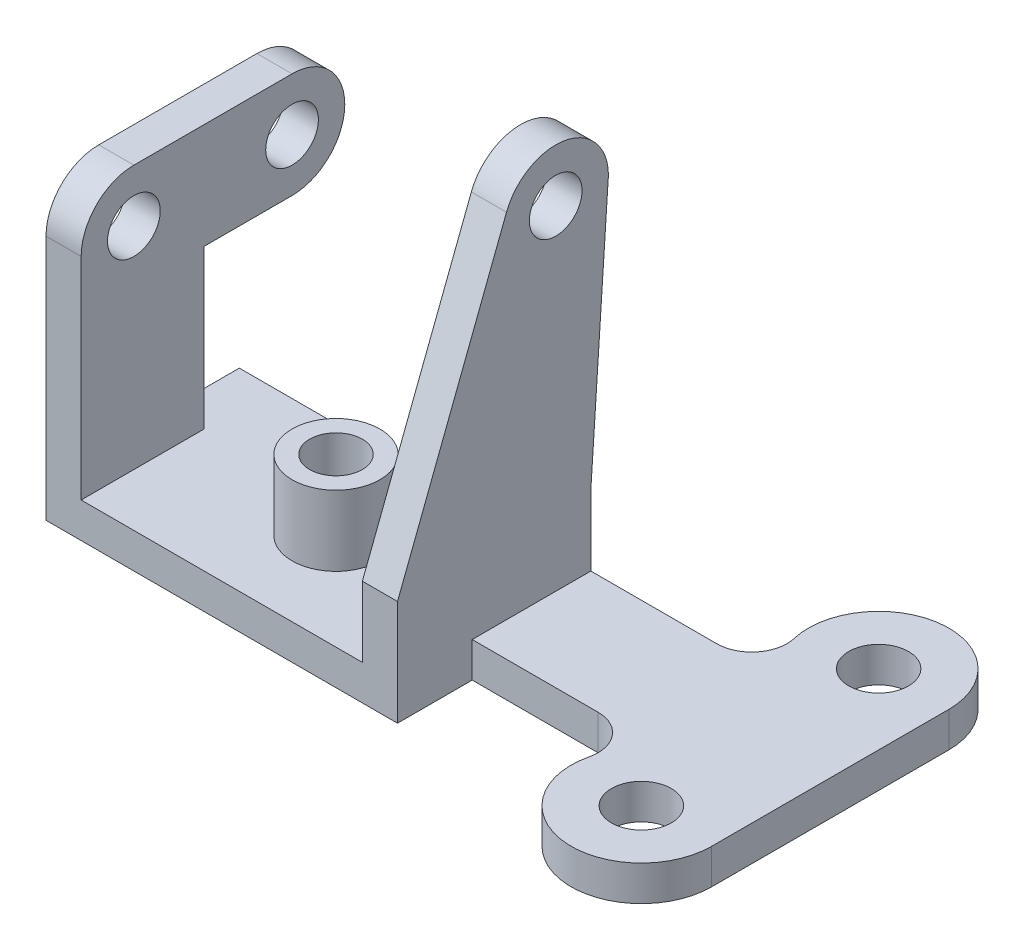
ISO-10303-21;
HEADER;
FILE_DESCRIPTION(('STEP AP214'),'2;1');
FILE_NAME('part.step','',(''),(''),'','','');
FILE_SCHEMA(('AUTOMOTIVE_DESIGN { 1 0 10303 214 1 1 1 1 }'));
ENDSEC;
DATA;
#1=APPLICATION_CONTEXT('core data for automotive mechanical design processes');
#2=APPLICATION_PROTOCOL_DEFINITION('international standard','automotive_design',2000,#1);
#3=PRODUCT_CONTEXT('',#1,'mechanical');
#4=PRODUCT('Part','Part','',(#3));
#5=PRODUCT_RELATED_PRODUCT_CATEGORY('part','',(#4));
#6=PRODUCT_DEFINITION_FORMATION('','',#4);
#7=PRODUCT_DEFINITION_CONTEXT('part definition',#1,'design');
#8=PRODUCT_DEFINITION('design','',#6,#7);
#9=PRODUCT_DEFINITION_SHAPE('','',#8);
#10=(LENGTH_UNIT() NAMED_UNIT(*) SI_UNIT(.MILLI.,.METRE.));
#11=(NAMED_UNIT(*) PLANE_ANGLE_UNIT() SI_UNIT($,.RADIAN.));
#12=(NAMED_UNIT(*) SI_UNIT($,.STERADIAN.) SOLID_ANGLE_UNIT());
#13=UNCERTAINTY_MEASURE_WITH_UNIT(LENGTH_MEASURE(1.E-05),#10,'distance_accuracy_value','');
#14=(GEOMETRIC_REPRESENTATION_CONTEXT(3) GLOBAL_UNCERTAINTY_ASSIGNED_CONTEXT((#13)) GLOBAL_UNIT_ASSIGNED_CONTEXT((#10,
#11,#12)) REPRESENTATION_CONTEXT('',''));
#15=CARTESIAN_POINT('',(0.,0.,0.));
#16=DIRECTION('',(0.,0.,1.));
#17=DIRECTION('',(1.,0.,0.));
#18=AXIS2_PLACEMENT_3D('',#15,#16,#17);
#19=CARTESIAN_POINT('',(0.,20.,0.));
#20=DIRECTION('',(0.,1.,0.));
#21=DIRECTION('',(0.,0.,1.));
#22=AXIS2_PLACEMENT_3D('',#19,#20,#21);
#23=PLANE('',#22);
#24=CARTESIAN_POINT('',(9.99999999999997,20.,0.));
#25=DIRECTION('',(0.,1.,0.));
#26=DIRECTION('',(0.,0.,1.));
#27=AXIS2_PLACEMENT_3D('',#24,#25,#26);
#28=CIRCLE('',#27,25.);
#29=CARTESIAN_POINT('',(9.99999999999997,20.,25.));
#30=VERTEX_POINT('',#29);
#31=EDGE_CURVE('E805',#30,#30,#28,.T.);
#32=ORIENTED_EDGE('',*,*,#31,.F.);
#33=EDGE_LOOP('',(#32));
#34=FACE_BOUND('',#33,.T.);
#35=DIRECTION('',(1.,0.,0.));
#36=VECTOR('',#35,1.);
#37=CARTESIAN_POINT('',(-100.,20.,55.));
#38=LINE('',#37,#36);
#39=CARTESIAN_POINT('',(-80.,20.,55.));
#40=VERTEX_POINT('',#39);
#41=CARTESIAN_POINT('',(80.,20.,55.));
#42=VERTEX_POINT('',#41);
#43=EDGE_CURVE('E68',#40,#42,#38,.T.);
#44=ORIENTED_EDGE('',*,*,#43,.T.);
#45=DIRECTION('',(0.,0.,1.));
#46=VECTOR('',#45,1.);
#47=CARTESIAN_POINT('',(80.,20.,0.));
#48=LINE('',#47,#46);
#49=CARTESIAN_POINT('',(80.,20.,-55.));
#50=VERTEX_POINT('',#49);
#51=EDGE_CURVE('E61',#50,#42,#48,.T.);
#52=ORIENTED_EDGE('',*,*,#51,.F.);
#53=DIRECTION('',(-1.,0.,0.));
#54=VECTOR('',#53,1.);
#55=CARTESIAN_POINT('',(-100.,20.,-55.));
#56=LINE('',#55,#54);
#57=CARTESIAN_POINT('',(-100.,20.,-55.));
#58=VERTEX_POINT('',#57);
#59=EDGE_CURVE('E372',#50,#58,#56,.T.);
#60=ORIENTED_EDGE('',*,*,#59,.T.);
#61=DIRECTION('',(0.,0.,1.));
#62=VECTOR('',#61,1.);
#63=CARTESIAN_POINT('',(-100.,20.,-55.));
#64=LINE('',#63,#62);
#65=CARTESIAN_POINT('',(-100.,20.,-15.));
#66=VERTEX_POINT('',#65);
#67=EDGE_CURVE('E373',#58,#66,#64,.T.);
#68=ORIENTED_EDGE('',*,*,#67,.T.);
#69=DIRECTION('',(-1.,0.,0.));
#70=VECTOR('',#69,1.);
#71=CARTESIAN_POINT('',(0.,20.,-15.));
#72=LINE('',#71,#70);
#73=CARTESIAN_POINT('',(-80.,20.,-15.));
#74=VERTEX_POINT('',#73);
#75=EDGE_CURVE('E303',#74,#66,#72,.T.);
#76=ORIENTED_EDGE('',*,*,#75,.F.);
#77=DIRECTION('',(0.,0.,1.));
#78=VECTOR('',#77,1.);
#79=CARTESIAN_POINT('',(-80.,20.,0.));
#80=LINE('',#79,#78);
#81=EDGE_CURVE('E291',#74,#40,#80,.T.);
#82=ORIENTED_EDGE('',*,*,#81,.T.);
#83=EDGE_LOOP('',(#44,#52,#60,#68,#76,#82));
#84=FACE_BOUND('',#83,.T.);
#85=ADVANCED_FACE('F50',(#34,#84),#23,.T.);
#86=CARTESIAN_POINT('',(100.,20.,-55.));
#87=DIRECTION('',(-1.,0.,0.));
#88=DIRECTION('',(0.,0.,1.));
#89=AXIS2_PLACEMENT_3D('',#86,#87,#88);
#90=PLANE('',#89);
#91=DIRECTION('',(0.,0.,-1.));
#92=VECTOR('',#91,1.);
#93=CARTESIAN_POINT('',(100.,0.,-55.));
#94=LINE('',#93,#92);
#95=CARTESIAN_POINT('',(100.,0.,55.));
#96=VERTEX_POINT('',#95);
#97=CARTESIAN_POINT('',(100.,0.,12.5));
#98=VERTEX_POINT('',#97);
#99=EDGE_CURVE('E358',#96,#98,#94,.T.);
#100=ORIENTED_EDGE('',*,*,#99,.T.);
#101=DIRECTION('',(0.,1.,0.));
#102=VECTOR('',#101,1.);
#103=CARTESIAN_POINT('',(100.,0.,12.5));
#104=LINE('',#103,#102);
#105=CARTESIAN_POINT('',(100.,20.,12.5));
#106=VERTEX_POINT('',#105);
#107=EDGE_CURVE('E336',#98,#106,#104,.T.);
#108=ORIENTED_EDGE('',*,*,#107,.T.);
#109=DIRECTION('',(0.,0.,1.));
#110=VECTOR('',#109,1.);
#111=CARTESIAN_POINT('',(100.,20.,0.));
#112=LINE('',#111,#110);
#113=CARTESIAN_POINT('',(100.,20.,-55.));
#114=VERTEX_POINT('',#113);
#115=EDGE_CURVE('E240',#114,#106,#112,.T.);
#116=ORIENTED_EDGE('',*,*,#115,.F.);
#117=DIRECTION('',(0.,1.,0.));
#118=VECTOR('',#117,1.);
#119=CARTESIAN_POINT('',(100.,0.,-55.));
#120=LINE('',#119,#118);
#121=CARTESIAN_POINT('',(100.,60.,-55.));
#122=VERTEX_POINT('',#121);
#123=EDGE_CURVE('E217',#114,#122,#120,.T.);
#124=ORIENTED_EDGE('',*,*,#123,.T.);
#125=DIRECTION('',(0.,0.997785157856609,-0.0665190105237738));
#126=VECTOR('',#125,1.);
#127=CARTESIAN_POINT('',(100.,-3.38495575221238,-50.7743362831858));
#128=LINE('',#127,#126);
#129=CARTESIAN_POINT('',(100.,210.,-65.));
#130=VERTEX_POINT('',#129);
#131=EDGE_CURVE('E227',#122,#130,#128,.T.);
#132=ORIENTED_EDGE('',*,*,#131,.T.);
#133=CARTESIAN_POINT('',(100.,210.,-35.));
#134=DIRECTION('',(1.,0.,0.));
#135=DIRECTION('',(0.,0.,-1.));
#136=AXIS2_PLACEMENT_3D('',#133,#134,#135);
#137=CIRCLE('',#136,30.);
#138=CARTESIAN_POINT('',(100.,220.794430534954,-7.00928244174394));
#139=VERTEX_POINT('',#138);
#140=EDGE_CURVE('E194',#130,#139,#137,.T.);
#141=ORIENTED_EDGE('',*,*,#140,.T.);
#142=DIRECTION('',(0.,0.933023918608534,-0.35981435116512));
#143=VECTOR('',#142,1.);
#144=CARTESIAN_POINT('',(100.,26.2323288125243,68.0222735519993));
#145=LINE('',#144,#143);
#146=CARTESIAN_POINT('',(100.,60.,55.));
#147=VERTEX_POINT('',#146);
#148=EDGE_CURVE('E232',#147,#139,#145,.T.);
#149=ORIENTED_EDGE('',*,*,#148,.F.);
#150=DIRECTION('',(0.,-1.,0.));
#151=VECTOR('',#150,1.);
#152=CARTESIAN_POINT('',(100.,20.,55.));
#153=LINE('',#152,#151);
#154=EDGE_CURVE('E380',#147,#96,#153,.T.);
#155=ORIENTED_EDGE('',*,*,#154,.T.);
#156=EDGE_LOOP('',(#100,#108,#116,#124,#132,#141,#149,#155));
#157=FACE_BOUND('',#156,.T.);
#158=CARTESIAN_POINT('',(100.,210.,-35.));
#159=DIRECTION('',(1.,0.,0.));
#160=DIRECTION('',(0.,0.,-1.));
#161=AXIS2_PLACEMENT_3D('',#158,#159,#160);
#162=CIRCLE('',#161,15.);
#163=CARTESIAN_POINT('',(100.,210.,-50.));
#164=VERTEX_POINT('',#163);
#165=EDGE_CURVE('E230',#164,#164,#162,.T.);
#166=ORIENTED_EDGE('',*,*,#165,.F.);
#167=EDGE_LOOP('',(#166));
#168=FACE_BOUND('',#167,.T.);
#169=ADVANCED_FACE('F47',(#157,#168),#90,.F.);
#170=CARTESIAN_POINT('',(-100.,20.,-55.));
#171=DIRECTION('',(0.,0.,1.));
#172=DIRECTION('',(1.,0.,0.));
#173=AXIS2_PLACEMENT_3D('',#170,#171,#172);
#174=PLANE('',#173);
#175=DIRECTION('',(-1.,0.,0.));
#176=VECTOR('',#175,1.);
#177=CARTESIAN_POINT('',(-100.,0.,-55.));
#178=LINE('',#177,#176);
#179=CARTESIAN_POINT('',(171.596768068882,0.,-55.));
#180=VERTEX_POINT('',#179);
#181=CARTESIAN_POINT('',(-100.,0.,-55.));
#182=VERTEX_POINT('',#181);
#183=EDGE_CURVE('E379',#180,#182,#178,.T.);
#184=ORIENTED_EDGE('',*,*,#183,.T.);
#185=DIRECTION('',(0.,-1.,0.));
#186=VECTOR('',#185,1.);
#187=CARTESIAN_POINT('',(-100.,20.,-55.));
#188=LINE('',#187,#186);
#189=EDGE_CURVE('E11',#58,#182,#188,.T.);
#190=ORIENTED_EDGE('',*,*,#189,.F.);
#191=ORIENTED_EDGE('',*,*,#59,.F.);
#192=DIRECTION('',(0.,1.,0.));
#193=VECTOR('',#192,1.);
#194=CARTESIAN_POINT('',(80.,0.,-55.));
#195=LINE('',#194,#193);
#196=CARTESIAN_POINT('',(80.,60.,-55.));
#197=VERTEX_POINT('',#196);
#198=EDGE_CURVE('E203',#50,#197,#195,.T.);
#199=ORIENTED_EDGE('',*,*,#198,.T.);
#200=DIRECTION('',(1.,0.,0.));
#201=VECTOR('',#200,1.);
#202=CARTESIAN_POINT('',(80.,60.,-55.));
#203=LINE('',#202,#201);
#204=EDGE_CURVE('E212',#197,#122,#203,.T.);
#205=ORIENTED_EDGE('',*,*,#204,.T.);
#206=ORIENTED_EDGE('',*,*,#123,.F.);
#207=CARTESIAN_POINT('',(171.596768068882,20.,-55.));
#208=VERTEX_POINT('',#207);
#209=EDGE_CURVE('E371',#208,#114,#56,.T.);
#210=ORIENTED_EDGE('',*,*,#209,.F.);
#211=DIRECTION('',(0.,1.,0.));
#212=VECTOR('',#211,1.);
#213=CARTESIAN_POINT('',(171.596768068882,0.,-55.));
#214=LINE('',#213,#212);
#215=EDGE_CURVE('E352',#180,#208,#214,.T.);
#216=ORIENTED_EDGE('',*,*,#215,.F.);
#217=EDGE_LOOP('',(#184,#190,#191,#199,#205,#206,#210,#216));
#218=FACE_BOUND('',#217,.T.);
#219=ADVANCED_FACE('F407',(#218),#174,.F.);
#220=CARTESIAN_POINT('',(-100.,20.,-55.));
#221=DIRECTION('',(1.,0.,0.));
#222=DIRECTION('',(0.,0.,-1.));
#223=AXIS2_PLACEMENT_3D('',#220,#221,#222);
#224=PLANE('',#223);
#225=DIRECTION('',(0.,0.,1.));
#226=VECTOR('',#225,1.);
#227=CARTESIAN_POINT('',(-100.,0.,-55.));
#228=LINE('',#227,#226);
#229=CARTESIAN_POINT('',(-100.,0.,55.));
#230=VERTEX_POINT('',#229);
#231=EDGE_CURVE('E385',#182,#230,#228,.T.);
#232=ORIENTED_EDGE('',*,*,#231,.T.);
#233=DIRECTION('',(0.,-1.,0.));
#234=VECTOR('',#233,1.);
#235=CARTESIAN_POINT('',(-100.,20.,55.));
#236=LINE('',#235,#234);
#237=CARTESIAN_POINT('',(-100.,140.,55.));
#238=VERTEX_POINT('',#237);
#239=EDGE_CURVE('E57',#238,#230,#236,.T.);
#240=ORIENTED_EDGE('',*,*,#239,.F.);
#241=CARTESIAN_POINT('',(-100.,140.,25.));
#242=DIRECTION('',(-1.,0.,0.));
#243=DIRECTION('',(0.,0.,1.));
#244=AXIS2_PLACEMENT_3D('',#241,#242,#243);
#245=CIRCLE('',#244,30.);
#246=CARTESIAN_POINT('',(-100.,170.,25.));
#247=VERTEX_POINT('',#246);
#248=EDGE_CURVE('E253',#238,#247,#245,.T.);
#249=ORIENTED_EDGE('',*,*,#248,.T.);
#250=DIRECTION('',(0.,0.,1.));
#251=VECTOR('',#250,1.);
#252=CARTESIAN_POINT('',(-100.,170.,0.));
#253=LINE('',#252,#251);
#254=CARTESIAN_POINT('',(-100.,170.,-65.));
#255=VERTEX_POINT('',#254);
#256=EDGE_CURVE('E280',#255,#247,#253,.T.);
#257=ORIENTED_EDGE('',*,*,#256,.F.);
#258=CARTESIAN_POINT('',(-100.,140.,-65.));
#259=DIRECTION('',(-1.,0.,0.));
#260=DIRECTION('',(0.,0.,1.));
#261=AXIS2_PLACEMENT_3D('',#258,#259,#260);
#262=CIRCLE('',#261,30.);
#263=CARTESIAN_POINT('',(-100.,110.,-65.));
#264=VERTEX_POINT('',#263);
#265=EDGE_CURVE('E278',#255,#264,#262,.T.);
#266=ORIENTED_EDGE('',*,*,#265,.T.);
#267=DIRECTION('',(0.,0.,1.));
#268=VECTOR('',#267,1.);
#269=CARTESIAN_POINT('',(-100.,110.,0.));
#270=LINE('',#269,#268);
#271=CARTESIAN_POINT('',(-100.,110.,-15.));
#272=VERTEX_POINT('',#271);
#273=EDGE_CURVE('E281',#264,#272,#270,.T.);
#274=ORIENTED_EDGE('',*,*,#273,.T.);
#275=DIRECTION('',(0.,-1.,0.));
#276=VECTOR('',#275,1.);
#277=CARTESIAN_POINT('',(-100.,0.,-15.));
#278=LINE('',#277,#276);
#279=EDGE_CURVE('E286',#272,#66,#278,.T.);
#280=ORIENTED_EDGE('',*,*,#279,.T.);
#281=ORIENTED_EDGE('',*,*,#67,.F.);
#282=ORIENTED_EDGE('',*,*,#189,.T.);
#283=EDGE_LOOP('',(#232,#240,#249,#257,#266,#274,#280,#281,#282));
#284=FACE_BOUND('',#283,.T.);
#285=CARTESIAN_POINT('',(-100.,140.,25.));
#286=DIRECTION('',(-1.,0.,0.));
#287=DIRECTION('',(0.,0.,1.));
#288=AXIS2_PLACEMENT_3D('',#285,#286,#287);
#289=CIRCLE('',#288,15.);
#290=CARTESIAN_POINT('',(-100.,140.,40.));
#291=VERTEX_POINT('',#290);
#292=EDGE_CURVE('E245',#291,#291,#289,.T.);
#293=ORIENTED_EDGE('',*,*,#292,.F.);
#294=EDGE_LOOP('',(#293));
#295=FACE_BOUND('',#294,.T.);
#296=CARTESIAN_POINT('',(-100.,140.,-65.));
#297=DIRECTION('',(-1.,0.,0.));
#298=DIRECTION('',(0.,0.,1.));
#299=AXIS2_PLACEMENT_3D('',#296,#297,#298);
#300=CIRCLE('',#299,15.);
#301=CARTESIAN_POINT('',(-100.,140.,-50.));
#302=VERTEX_POINT('',#301);
#303=EDGE_CURVE('E273',#302,#302,#300,.T.);
#304=ORIENTED_EDGE('',*,*,#303,.F.);
#305=EDGE_LOOP('',(#304));
#306=FACE_BOUND('',#305,.T.);
#307=ADVANCED_FACE('F420',(#284,#295,#306),#224,.F.);
#308=CARTESIAN_POINT('',(-100.,20.,55.));
#309=DIRECTION('',(0.,0.,-1.));
#310=DIRECTION('',(-1.,0.,0.));
#311=AXIS2_PLACEMENT_3D('',#308,#309,#310);
#312=PLANE('',#311);
#313=DIRECTION('',(1.,0.,0.));
#314=VECTOR('',#313,1.);
#315=CARTESIAN_POINT('',(-100.,0.,55.));
#316=LINE('',#315,#314);
#317=EDGE_CURVE('E383',#230,#96,#316,.T.);
#318=ORIENTED_EDGE('',*,*,#317,.T.);
#319=ORIENTED_EDGE('',*,*,#154,.F.);
#320=DIRECTION('',(1.,0.,0.));
#321=VECTOR('',#320,1.);
#322=CARTESIAN_POINT('',(80.,60.,55.));
#323=LINE('',#322,#321);
#324=CARTESIAN_POINT('',(80.,60.,55.));
#325=VERTEX_POINT('',#324);
#326=EDGE_CURVE('E241',#325,#147,#323,.T.);
#327=ORIENTED_EDGE('',*,*,#326,.F.);
#328=DIRECTION('',(0.,1.,0.));
#329=VECTOR('',#328,1.);
#330=CARTESIAN_POINT('',(80.,0.,55.));
#331=LINE('',#330,#329);
#332=EDGE_CURVE('E224',#42,#325,#331,.T.);
#333=ORIENTED_EDGE('',*,*,#332,.F.);
#334=ORIENTED_EDGE('',*,*,#43,.F.);
#335=DIRECTION('',(0.,-1.,0.));
#336=VECTOR('',#335,1.);
#337=CARTESIAN_POINT('',(-80.,0.,55.));
#338=LINE('',#337,#336);
#339=CARTESIAN_POINT('',(-80.,140.,55.));
#340=VERTEX_POINT('',#339);
#341=EDGE_CURVE('E264',#340,#40,#338,.T.);
#342=ORIENTED_EDGE('',*,*,#341,.F.);
#343=DIRECTION('',(-1.,0.,0.));
#344=VECTOR('',#343,1.);
#345=CARTESIAN_POINT('',(-80.,140.,55.));
#346=LINE('',#345,#344);
#347=EDGE_CURVE('E294',#340,#238,#346,.T.);
#348=ORIENTED_EDGE('',*,*,#347,.T.);
#349=ORIENTED_EDGE('',*,*,#239,.T.);
#350=EDGE_LOOP('',(#318,#319,#327,#333,#334,#342,#348,#349));
#351=FACE_BOUND('',#350,.T.);
#352=ADVANCED_FACE('F393',(#351),#312,.F.);
#353=ORIENTED_EDGE('',*,*,#115,.T.);
#354=DIRECTION('',(1.,0.,0.));
#355=VECTOR('',#354,1.);
#356=CARTESIAN_POINT('',(100.,20.,12.5));
#357=LINE('',#356,#355);
#358=CARTESIAN_POINT('',(171.596768068882,20.,12.5));
#359=VERTEX_POINT('',#358);
#360=EDGE_CURVE('E316',#106,#359,#357,.T.);
#361=ORIENTED_EDGE('',*,*,#360,.T.);
#362=CARTESIAN_POINT('',(171.596768068882,20.,32.5));
#363=DIRECTION('',(0.,-1.,0.));
#364=DIRECTION('',(0.,0.,-1.));
#365=AXIS2_PLACEMENT_3D('',#362,#363,#364);
#366=CIRCLE('',#365,20.);
#367=CARTESIAN_POINT('',(191.064512045921,20.,37.0833333333333));
#368=VERTEX_POINT('',#367);
#369=EDGE_CURVE('E341',#359,#368,#366,.T.);
#370=ORIENTED_EDGE('',*,*,#369,.T.);
#371=CARTESIAN_POINT('',(230.,20.,46.25));
#372=DIRECTION('',(0.,1.,0.));
#373=DIRECTION('',(0.,0.,1.));
#374=AXIS2_PLACEMENT_3D('',#371,#372,#373);
#375=CIRCLE('',#374,40.);
#376=CARTESIAN_POINT('',(270.,20.,46.25));
#377=VERTEX_POINT('',#376);
#378=EDGE_CURVE('E342',#368,#377,#375,.T.);
#379=ORIENTED_EDGE('',*,*,#378,.T.);
#380=DIRECTION('',(0.,0.,-1.));
#381=VECTOR('',#380,1.);
#382=CARTESIAN_POINT('',(270.,20.,-88.75));
#383=LINE('',#382,#381);
#384=CARTESIAN_POINT('',(270.,20.,-88.75));
#385=VERTEX_POINT('',#384);
#386=EDGE_CURVE('E350',#377,#385,#383,.T.);
#387=ORIENTED_EDGE('',*,*,#386,.T.);
#388=CARTESIAN_POINT('',(230.,20.,-88.75));
#389=DIRECTION('',(0.,1.,0.));
#390=DIRECTION('',(0.,0.,1.));
#391=AXIS2_PLACEMENT_3D('',#388,#389,#390);
#392=CIRCLE('',#391,40.);
#393=CARTESIAN_POINT('',(191.064512045921,20.,-79.5833333333334));
#394=VERTEX_POINT('',#393);
#395=EDGE_CURVE('E348',#385,#394,#392,.T.);
#396=ORIENTED_EDGE('',*,*,#395,.T.);
#397=CARTESIAN_POINT('',(171.596768068882,20.,-75.));
#398=DIRECTION('',(0.,-1.,0.));
#399=DIRECTION('',(0.,0.,1.));
#400=AXIS2_PLACEMENT_3D('',#397,#398,#399);
#401=CIRCLE('',#400,20.);
#402=EDGE_CURVE('E323',#394,#208,#401,.T.);
#403=ORIENTED_EDGE('',*,*,#402,.T.);
#404=ORIENTED_EDGE('',*,*,#209,.T.);
#405=EDGE_LOOP('',(#353,#361,#370,#379,#387,#396,#403,#404));
#406=FACE_BOUND('',#405,.T.);
#407=CARTESIAN_POINT('',(230.,20.,46.25));
#408=DIRECTION('',(0.,1.,0.));
#409=DIRECTION('',(0.,0.,1.));
#410=AXIS2_PLACEMENT_3D('',#407,#408,#409);
#411=CIRCLE('',#410,17.);
#412=CARTESIAN_POINT('',(230.,20.,63.25));
#413=VERTEX_POINT('',#412);
#414=EDGE_CURVE('E308',#413,#413,#411,.T.);
#415=ORIENTED_EDGE('',*,*,#414,.F.);
#416=EDGE_LOOP('',(#415));
#417=FACE_BOUND('',#416,.T.);
#418=CARTESIAN_POINT('',(230.,20.,-88.75));
#419=DIRECTION('',(0.,1.,0.));
#420=DIRECTION('',(0.,0.,1.));
#421=AXIS2_PLACEMENT_3D('',#418,#419,#420);
#422=CIRCLE('',#421,17.);
#423=CARTESIAN_POINT('',(230.,20.,-71.75));
#424=VERTEX_POINT('',#423);
#425=EDGE_CURVE('E309',#424,#424,#422,.T.);
#426=ORIENTED_EDGE('',*,*,#425,.F.);
#427=EDGE_LOOP('',(#426));
#428=FACE_BOUND('',#427,.T.);
#429=ADVANCED_FACE('F460',(#406,#417,#428),#23,.T.);
#430=CARTESIAN_POINT('',(0.,0.,0.));
#431=DIRECTION('',(0.,1.,0.));
#432=DIRECTION('',(0.,0.,1.));
#433=AXIS2_PLACEMENT_3D('',#430,#431,#432);
#434=PLANE('',#433);
#435=CARTESIAN_POINT('',(9.99999999999997,0.,0.));
#436=DIRECTION('',(0.,1.,0.));
#437=DIRECTION('',(0.,0.,1.));
#438=AXIS2_PLACEMENT_3D('',#435,#436,#437);
#439=CIRCLE('',#438,15.);
#440=CARTESIAN_POINT('',(9.99999999999997,0.,15.));
#441=VERTEX_POINT('',#440);
#442=EDGE_CURVE('E51',#441,#441,#439,.T.);
#443=ORIENTED_EDGE('',*,*,#442,.T.);
#444=EDGE_LOOP('',(#443));
#445=FACE_BOUND('',#444,.T.);
#446=ORIENTED_EDGE('',*,*,#317,.F.);
#447=ORIENTED_EDGE('',*,*,#231,.F.);
#448=ORIENTED_EDGE('',*,*,#183,.F.);
#449=CARTESIAN_POINT('',(171.596768068882,0.,-75.));
#450=DIRECTION('',(0.,-1.,0.));
#451=DIRECTION('',(0.,0.,1.));
#452=AXIS2_PLACEMENT_3D('',#449,#450,#451);
#453=CIRCLE('',#452,20.);
#454=CARTESIAN_POINT('',(191.064512045921,0.,-79.5833333333334));
#455=VERTEX_POINT('',#454);
#456=EDGE_CURVE('E333',#455,#180,#453,.T.);
#457=ORIENTED_EDGE('',*,*,#456,.F.);
#458=CARTESIAN_POINT('',(230.,0.,-88.75));
#459=DIRECTION('',(0.,1.,0.));
#460=DIRECTION('',(0.,0.,1.));
#461=AXIS2_PLACEMENT_3D('',#458,#459,#460);
#462=CIRCLE('',#461,40.);
#463=CARTESIAN_POINT('',(270.,0.,-88.75));
#464=VERTEX_POINT('',#463);
#465=EDGE_CURVE('E335',#464,#455,#462,.T.);
#466=ORIENTED_EDGE('',*,*,#465,.F.);
#467=DIRECTION('',(0.,0.,-1.));
#468=VECTOR('',#467,1.);
#469=CARTESIAN_POINT('',(270.,0.,-88.75));
#470=LINE('',#469,#468);
#471=CARTESIAN_POINT('',(270.,0.,46.25));
#472=VERTEX_POINT('',#471);
#473=EDGE_CURVE('E328',#472,#464,#470,.T.);
#474=ORIENTED_EDGE('',*,*,#473,.F.);
#475=CARTESIAN_POINT('',(230.,0.,46.25));
#476=DIRECTION('',(0.,1.,0.));
#477=DIRECTION('',(0.,0.,1.));
#478=AXIS2_PLACEMENT_3D('',#475,#476,#477);
#479=CIRCLE('',#478,40.);
#480=CARTESIAN_POINT('',(191.064512045921,0.,37.0833333333333));
#481=VERTEX_POINT('',#480);
#482=EDGE_CURVE('E326',#481,#472,#479,.T.);
#483=ORIENTED_EDGE('',*,*,#482,.F.);
#484=CARTESIAN_POINT('',(171.596768068882,0.,32.5));
#485=DIRECTION('',(0.,-1.,0.));
#486=DIRECTION('',(0.,0.,-1.));
#487=AXIS2_PLACEMENT_3D('',#484,#485,#486);
#488=CIRCLE('',#487,20.);
#489=CARTESIAN_POINT('',(171.596768068882,0.,12.5));
#490=VERTEX_POINT('',#489);
#491=EDGE_CURVE('E325',#490,#481,#488,.T.);
#492=ORIENTED_EDGE('',*,*,#491,.F.);
#493=DIRECTION('',(1.,0.,0.));
#494=VECTOR('',#493,1.);
#495=CARTESIAN_POINT('',(100.,0.,12.5));
#496=LINE('',#495,#494);
#497=EDGE_CURVE('E317',#98,#490,#496,.T.);
#498=ORIENTED_EDGE('',*,*,#497,.F.);
#499=ORIENTED_EDGE('',*,*,#99,.F.);
#500=EDGE_LOOP('',(#446,#447,#448,#457,#466,#474,#483,#492,#498,#499));
#501=FACE_BOUND('',#500,.T.);
#502=CARTESIAN_POINT('',(230.,0.,46.25));
#503=DIRECTION('',(0.,1.,0.));
#504=DIRECTION('',(0.,0.,1.));
#505=AXIS2_PLACEMENT_3D('',#502,#503,#504);
#506=CIRCLE('',#505,17.);
#507=CARTESIAN_POINT('',(230.,0.,63.25));
#508=VERTEX_POINT('',#507);
#509=EDGE_CURVE('E307',#508,#508,#506,.T.);
#510=ORIENTED_EDGE('',*,*,#509,.T.);
#511=EDGE_LOOP('',(#510));
#512=FACE_BOUND('',#511,.T.);
#513=CARTESIAN_POINT('',(230.,0.,-88.75));
#514=DIRECTION('',(0.,1.,0.));
#515=DIRECTION('',(0.,0.,1.));
#516=AXIS2_PLACEMENT_3D('',#513,#514,#515);
#517=CIRCLE('',#516,17.);
#518=CARTESIAN_POINT('',(230.,0.,-71.75));
#519=VERTEX_POINT('',#518);
#520=EDGE_CURVE('E311',#519,#519,#517,.T.);
#521=ORIENTED_EDGE('',*,*,#520,.T.);
#522=EDGE_LOOP('',(#521));
#523=FACE_BOUND('',#522,.T.);
#524=ADVANCED_FACE('F398',(#445,#501,#512,#523),#434,.F.);
#525=CARTESIAN_POINT('',(171.596768068882,0.,-75.));
#526=DIRECTION('',(0.,1.,0.));
#527=DIRECTION('',(0.,0.,1.));
#528=AXIS2_PLACEMENT_3D('',#525,#526,#527);
#529=CYLINDRICAL_SURFACE('',#528,20.);
#530=ORIENTED_EDGE('',*,*,#402,.F.);
#531=DIRECTION('',(0.,1.,0.));
#532=VECTOR('',#531,1.);
#533=CARTESIAN_POINT('',(191.064512045921,0.,-79.5833333333334));
#534=LINE('',#533,#532);
#535=EDGE_CURVE('E357',#455,#394,#534,.T.);
#536=ORIENTED_EDGE('',*,*,#535,.F.);
#537=ORIENTED_EDGE('',*,*,#456,.T.);
#538=ORIENTED_EDGE('',*,*,#215,.T.);
#539=EDGE_LOOP('',(#530,#536,#537,#538));
#540=FACE_BOUND('',#539,.T.);
#541=ADVANCED_FACE('F471',(#540),#529,.F.);
#542=CARTESIAN_POINT('',(230.,0.,-88.75));
#543=DIRECTION('',(0.,1.,0.));
#544=DIRECTION('',(0.,0.,1.));
#545=AXIS2_PLACEMENT_3D('',#542,#543,#544);
#546=CYLINDRICAL_SURFACE('',#545,40.);
#547=ORIENTED_EDGE('',*,*,#395,.F.);
#548=DIRECTION('',(0.,1.,0.));
#549=VECTOR('',#548,1.);
#550=CARTESIAN_POINT('',(270.,0.,-88.75));
#551=LINE('',#550,#549);
#552=EDGE_CURVE('E363',#464,#385,#551,.T.);
#553=ORIENTED_EDGE('',*,*,#552,.F.);
#554=ORIENTED_EDGE('',*,*,#465,.T.);
#555=ORIENTED_EDGE('',*,*,#535,.T.);
#556=EDGE_LOOP('',(#547,#553,#554,#555));
#557=FACE_BOUND('',#556,.T.);
#558=ADVANCED_FACE('F494',(#557),#546,.T.);
#559=CARTESIAN_POINT('',(270.,0.,-88.75));
#560=DIRECTION('',(1.,0.,0.));
#561=DIRECTION('',(0.,0.,-1.));
#562=AXIS2_PLACEMENT_3D('',#559,#560,#561);
#563=PLANE('',#562);
#564=ORIENTED_EDGE('',*,*,#386,.F.);
#565=DIRECTION('',(0.,1.,0.));
#566=VECTOR('',#565,1.);
#567=CARTESIAN_POINT('',(270.,0.,46.25));
#568=LINE('',#567,#566);
#569=EDGE_CURVE('E361',#472,#377,#568,.T.);
#570=ORIENTED_EDGE('',*,*,#569,.F.);
#571=ORIENTED_EDGE('',*,*,#473,.T.);
#572=ORIENTED_EDGE('',*,*,#552,.T.);
#573=EDGE_LOOP('',(#564,#570,#571,#572));
#574=FACE_BOUND('',#573,.T.);
#575=ADVANCED_FACE('F496',(#574),#563,.T.);
#576=CARTESIAN_POINT('',(230.,0.,46.25));
#577=DIRECTION('',(0.,1.,0.));
#578=DIRECTION('',(0.,0.,1.));
#579=AXIS2_PLACEMENT_3D('',#576,#577,#578);
#580=CYLINDRICAL_SURFACE('',#579,40.);
#581=ORIENTED_EDGE('',*,*,#378,.F.);
#582=DIRECTION('',(0.,1.,0.));
#583=VECTOR('',#582,1.);
#584=CARTESIAN_POINT('',(191.064512045921,0.,37.0833333333333));
#585=LINE('',#584,#583);
#586=EDGE_CURVE('E364',#481,#368,#585,.T.);
#587=ORIENTED_EDGE('',*,*,#586,.F.);
#588=ORIENTED_EDGE('',*,*,#482,.T.);
#589=ORIENTED_EDGE('',*,*,#569,.T.);
#590=EDGE_LOOP('',(#581,#587,#588,#589));
#591=FACE_BOUND('',#590,.T.);
#592=ADVANCED_FACE('F501',(#591),#580,.T.);
#593=CARTESIAN_POINT('',(171.596768068882,0.,32.5));
#594=DIRECTION('',(0.,1.,0.));
#595=DIRECTION('',(0.,0.,1.));
#596=AXIS2_PLACEMENT_3D('',#593,#594,#595);
#597=CYLINDRICAL_SURFACE('',#596,20.);
#598=ORIENTED_EDGE('',*,*,#369,.F.);
#599=DIRECTION('',(0.,1.,0.));
#600=VECTOR('',#599,1.);
#601=CARTESIAN_POINT('',(171.596768068882,0.,12.5));
#602=LINE('',#601,#600);
#603=EDGE_CURVE('E370',#490,#359,#602,.T.);
#604=ORIENTED_EDGE('',*,*,#603,.F.);
#605=ORIENTED_EDGE('',*,*,#491,.T.);
#606=ORIENTED_EDGE('',*,*,#586,.T.);
#607=EDGE_LOOP('',(#598,#604,#605,#606));
#608=FACE_BOUND('',#607,.T.);
#609=ADVANCED_FACE('F488',(#608),#597,.F.);
#610=CARTESIAN_POINT('',(100.,0.,12.5));
#611=DIRECTION('',(0.,0.,1.));
#612=DIRECTION('',(1.,0.,0.));
#613=AXIS2_PLACEMENT_3D('',#610,#611,#612);
#614=PLANE('',#613);
#615=ORIENTED_EDGE('',*,*,#360,.F.);
#616=ORIENTED_EDGE('',*,*,#107,.F.);
#617=ORIENTED_EDGE('',*,*,#497,.T.);
#618=ORIENTED_EDGE('',*,*,#603,.T.);
#619=EDGE_LOOP('',(#615,#616,#617,#618));
#620=FACE_BOUND('',#619,.T.);
#621=ADVANCED_FACE('F483',(#620),#614,.T.);
#622=CARTESIAN_POINT('',(230.,0.,-88.75));
#623=DIRECTION('',(0.,1.,0.));
#624=DIRECTION('',(0.,0.,1.));
#625=AXIS2_PLACEMENT_3D('',#622,#623,#624);
#626=CYLINDRICAL_SURFACE('',#625,17.);
#627=ORIENTED_EDGE('',*,*,#520,.F.);
#628=EDGE_LOOP('',(#627));
#629=FACE_BOUND('',#628,.T.);
#630=ORIENTED_EDGE('',*,*,#425,.T.);
#631=EDGE_LOOP('',(#630));
#632=FACE_BOUND('',#631,.T.);
#633=ADVANCED_FACE('F449',(#629,#632),#626,.F.);
#634=CARTESIAN_POINT('',(230.,0.,46.25));
#635=DIRECTION('',(0.,1.,0.));
#636=DIRECTION('',(0.,0.,1.));
#637=AXIS2_PLACEMENT_3D('',#634,#635,#636);
#638=CYLINDRICAL_SURFACE('',#637,17.);
#639=ORIENTED_EDGE('',*,*,#509,.F.);
#640=EDGE_LOOP('',(#639));
#641=FACE_BOUND('',#640,.T.);
#642=ORIENTED_EDGE('',*,*,#414,.T.);
#643=EDGE_LOOP('',(#642));
#644=FACE_BOUND('',#643,.T.);
#645=ADVANCED_FACE('F442',(#641,#644),#638,.F.);
#646=CARTESIAN_POINT('',(-80.,170.,0.));
#647=DIRECTION('',(0.,-1.,0.));
#648=DIRECTION('',(0.,0.,-1.));
#649=AXIS2_PLACEMENT_3D('',#646,#647,#648);
#650=PLANE('',#649);
#651=ORIENTED_EDGE('',*,*,#256,.T.);
#652=DIRECTION('',(-1.,0.,0.));
#653=VECTOR('',#652,1.);
#654=CARTESIAN_POINT('',(-80.,170.,25.));
#655=LINE('',#654,#653);
#656=CARTESIAN_POINT('',(-80.,170.,25.));
#657=VERTEX_POINT('',#656);
#658=EDGE_CURVE('E292',#657,#247,#655,.T.);
#659=ORIENTED_EDGE('',*,*,#658,.F.);
#660=DIRECTION('',(0.,0.,1.));
#661=VECTOR('',#660,1.);
#662=CARTESIAN_POINT('',(-80.,170.,0.));
#663=LINE('',#662,#661);
#664=CARTESIAN_POINT('',(-80.,170.,-65.));
#665=VERTEX_POINT('',#664);
#666=EDGE_CURVE('E255',#665,#657,#663,.T.);
#667=ORIENTED_EDGE('',*,*,#666,.F.);
#668=DIRECTION('',(-1.,0.,0.));
#669=VECTOR('',#668,1.);
#670=CARTESIAN_POINT('',(-80.,170.,-65.));
#671=LINE('',#670,#669);
#672=EDGE_CURVE('E271',#665,#255,#671,.T.);
#673=ORIENTED_EDGE('',*,*,#672,.T.);
#674=EDGE_LOOP('',(#651,#659,#667,#673));
#675=FACE_BOUND('',#674,.T.);
#676=ADVANCED_FACE('F438',(#675),#650,.F.);
#677=CARTESIAN_POINT('',(-80.,140.,25.));
#678=DIRECTION('',(-1.,0.,0.));
#679=DIRECTION('',(0.,0.,1.));
#680=AXIS2_PLACEMENT_3D('',#677,#678,#679);
#681=CYLINDRICAL_SURFACE('',#680,30.);
#682=ORIENTED_EDGE('',*,*,#248,.F.);
#683=ORIENTED_EDGE('',*,*,#347,.F.);
#684=CARTESIAN_POINT('',(-80.,140.,25.));
#685=DIRECTION('',(-1.,0.,0.));
#686=DIRECTION('',(0.,0.,1.));
#687=AXIS2_PLACEMENT_3D('',#684,#685,#686);
#688=CIRCLE('',#687,30.);
#689=EDGE_CURVE('E268',#340,#657,#688,.T.);
#690=ORIENTED_EDGE('',*,*,#689,.T.);
#691=ORIENTED_EDGE('',*,*,#658,.T.);
#692=EDGE_LOOP('',(#682,#683,#690,#691));
#693=FACE_BOUND('',#692,.T.);
#694=ADVANCED_FACE('F434',(#693),#681,.T.);
#695=CARTESIAN_POINT('',(-80.,0.,-15.));
#696=DIRECTION('',(0.,0.,-1.));
#697=DIRECTION('',(-1.,0.,0.));
#698=AXIS2_PLACEMENT_3D('',#695,#696,#697);
#699=PLANE('',#698);
#700=DIRECTION('',(0.,-1.,0.));
#701=VECTOR('',#700,1.);
#702=CARTESIAN_POINT('',(-80.,0.,-15.));
#703=LINE('',#702,#701);
#704=CARTESIAN_POINT('',(-80.,110.,-15.));
#705=VERTEX_POINT('',#704);
#706=EDGE_CURVE('E265',#705,#74,#703,.T.);
#707=ORIENTED_EDGE('',*,*,#706,.T.);
#708=ORIENTED_EDGE('',*,*,#75,.T.);
#709=ORIENTED_EDGE('',*,*,#279,.F.);
#710=DIRECTION('',(-1.,0.,0.));
#711=VECTOR('',#710,1.);
#712=CARTESIAN_POINT('',(-80.,110.,-15.));
#713=LINE('',#712,#711);
#714=EDGE_CURVE('E300',#705,#272,#713,.T.);
#715=ORIENTED_EDGE('',*,*,#714,.F.);
#716=EDGE_LOOP('',(#707,#708,#709,#715));
#717=FACE_BOUND('',#716,.T.);
#718=ADVANCED_FACE('F417',(#717),#699,.T.);
#719=CARTESIAN_POINT('',(-80.,110.,0.));
#720=DIRECTION('',(0.,-1.,0.));
#721=DIRECTION('',(0.,0.,-1.));
#722=AXIS2_PLACEMENT_3D('',#719,#720,#721);
#723=PLANE('',#722);
#724=ORIENTED_EDGE('',*,*,#273,.F.);
#725=DIRECTION('',(-1.,0.,0.));
#726=VECTOR('',#725,1.);
#727=CARTESIAN_POINT('',(-80.,110.,-65.));
#728=LINE('',#727,#726);
#729=CARTESIAN_POINT('',(-80.,110.,-65.));
#730=VERTEX_POINT('',#729);
#731=EDGE_CURVE('E299',#730,#264,#728,.T.);
#732=ORIENTED_EDGE('',*,*,#731,.F.);
#733=DIRECTION('',(0.,0.,1.));
#734=VECTOR('',#733,1.);
#735=CARTESIAN_POINT('',(-80.,110.,0.));
#736=LINE('',#735,#734);
#737=EDGE_CURVE('E259',#730,#705,#736,.T.);
#738=ORIENTED_EDGE('',*,*,#737,.T.);
#739=ORIENTED_EDGE('',*,*,#714,.T.);
#740=EDGE_LOOP('',(#724,#732,#738,#739));
#741=FACE_BOUND('',#740,.T.);
#742=ADVANCED_FACE('F422',(#741),#723,.T.);
#743=CARTESIAN_POINT('',(-80.,140.,-65.));
#744=DIRECTION('',(-1.,0.,0.));
#745=DIRECTION('',(0.,0.,1.));
#746=AXIS2_PLACEMENT_3D('',#743,#744,#745);
#747=CYLINDRICAL_SURFACE('',#746,15.);
#748=CARTESIAN_POINT('',(-80.,140.,-65.));
#749=DIRECTION('',(-1.,0.,0.));
#750=DIRECTION('',(0.,0.,1.));
#751=AXIS2_PLACEMENT_3D('',#748,#749,#750);
#752=CIRCLE('',#751,15.);
#753=CARTESIAN_POINT('',(-80.,140.,-50.));
#754=VERTEX_POINT('',#753);
#755=EDGE_CURVE('E249',#754,#754,#752,.T.);
#756=ORIENTED_EDGE('',*,*,#755,.F.);
#757=EDGE_LOOP('',(#756));
#758=FACE_BOUND('',#757,.T.);
#759=ORIENTED_EDGE('',*,*,#303,.T.);
#760=EDGE_LOOP('',(#759));
#761=FACE_BOUND('',#760,.T.);
#762=ADVANCED_FACE('F594',(#758,#761),#747,.F.);
#763=CARTESIAN_POINT('',(-80.,140.,25.));
#764=DIRECTION('',(-1.,0.,0.));
#765=DIRECTION('',(0.,0.,1.));
#766=AXIS2_PLACEMENT_3D('',#763,#764,#765);
#767=CYLINDRICAL_SURFACE('',#766,15.);
#768=CARTESIAN_POINT('',(-80.,140.,25.));
#769=DIRECTION('',(-1.,0.,0.));
#770=DIRECTION('',(0.,0.,1.));
#771=AXIS2_PLACEMENT_3D('',#768,#769,#770);
#772=CIRCLE('',#771,15.);
#773=CARTESIAN_POINT('',(-80.,140.,40.));
#774=VERTEX_POINT('',#773);
#775=EDGE_CURVE('E250',#774,#774,#772,.T.);
#776=ORIENTED_EDGE('',*,*,#775,.F.);
#777=EDGE_LOOP('',(#776));
#778=FACE_BOUND('',#777,.T.);
#779=ORIENTED_EDGE('',*,*,#292,.T.);
#780=EDGE_LOOP('',(#779));
#781=FACE_BOUND('',#780,.T.);
#782=ADVANCED_FACE('F604',(#778,#781),#767,.F.);
#783=CARTESIAN_POINT('',(-80.,140.,-65.));
#784=DIRECTION('',(-1.,0.,0.));
#785=DIRECTION('',(0.,0.,1.));
#786=AXIS2_PLACEMENT_3D('',#783,#784,#785);
#787=CYLINDRICAL_SURFACE('',#786,30.);
#788=ORIENTED_EDGE('',*,*,#265,.F.);
#789=ORIENTED_EDGE('',*,*,#672,.F.);
#790=CARTESIAN_POINT('',(-80.,140.,-65.));
#791=DIRECTION('',(-1.,0.,0.));
#792=DIRECTION('',(0.,0.,1.));
#793=AXIS2_PLACEMENT_3D('',#790,#791,#792);
#794=CIRCLE('',#793,30.);
#795=EDGE_CURVE('E258',#665,#730,#794,.T.);
#796=ORIENTED_EDGE('',*,*,#795,.T.);
#797=ORIENTED_EDGE('',*,*,#731,.T.);
#798=EDGE_LOOP('',(#788,#789,#796,#797));
#799=FACE_BOUND('',#798,.T.);
#800=ADVANCED_FACE('F437',(#799),#787,.T.);
#801=CARTESIAN_POINT('',(-80.,0.,0.));
#802=DIRECTION('',(-1.,0.,0.));
#803=DIRECTION('',(0.,0.,1.));
#804=AXIS2_PLACEMENT_3D('',#801,#802,#803);
#805=PLANE('',#804);
#806=ORIENTED_EDGE('',*,*,#81,.F.);
#807=ORIENTED_EDGE('',*,*,#706,.F.);
#808=ORIENTED_EDGE('',*,*,#737,.F.);
#809=ORIENTED_EDGE('',*,*,#795,.F.);
#810=ORIENTED_EDGE('',*,*,#666,.T.);
#811=ORIENTED_EDGE('',*,*,#689,.F.);
#812=ORIENTED_EDGE('',*,*,#341,.T.);
#813=EDGE_LOOP('',(#806,#807,#808,#809,#810,#811,#812));
#814=FACE_BOUND('',#813,.T.);
#815=ORIENTED_EDGE('',*,*,#775,.T.);
#816=EDGE_LOOP('',(#815));
#817=FACE_BOUND('',#816,.T.);
#818=ORIENTED_EDGE('',*,*,#755,.T.);
#819=EDGE_LOOP('',(#818));
#820=FACE_BOUND('',#819,.T.);
#821=ADVANCED_FACE('F428',(#814,#817,#820),#805,.F.);
#822=CARTESIAN_POINT('',(80.,-3.38495575221238,-50.7743362831858));
#823=DIRECTION('',(0.,-0.0665190105237738,-0.997785157856609));
#824=DIRECTION('',(0.,0.997785157856609,-0.0665190105237738));
#825=AXIS2_PLACEMENT_3D('',#822,#823,#824);
#826=PLANE('',#825);
#827=ORIENTED_EDGE('',*,*,#131,.F.);
#828=ORIENTED_EDGE('',*,*,#204,.F.);
#829=DIRECTION('',(0.,0.997785157856609,-0.0665190105237738));
#830=VECTOR('',#829,1.);
#831=CARTESIAN_POINT('',(80.,-3.38495575221238,-50.7743362831858));
#832=LINE('',#831,#830);
#833=CARTESIAN_POINT('',(80.,210.,-65.));
#834=VERTEX_POINT('',#833);
#835=EDGE_CURVE('E210',#197,#834,#832,.T.);
#836=ORIENTED_EDGE('',*,*,#835,.T.);
#837=DIRECTION('',(1.,0.,0.));
#838=VECTOR('',#837,1.);
#839=CARTESIAN_POINT('',(80.,210.,-65.));
#840=LINE('',#839,#838);
#841=EDGE_CURVE('E187',#834,#130,#840,.T.);
#842=ORIENTED_EDGE('',*,*,#841,.T.);
#843=EDGE_LOOP('',(#827,#828,#836,#842));
#844=FACE_BOUND('',#843,.T.);
#845=ADVANCED_FACE('F213',(#844),#826,.T.);
#846=CARTESIAN_POINT('',(80.,26.2323288125243,68.0222735519993));
#847=DIRECTION('',(0.,-0.35981435116512,-0.933023918608534));
#848=DIRECTION('',(0.,0.933023918608534,-0.35981435116512));
#849=AXIS2_PLACEMENT_3D('',#846,#847,#848);
#850=PLANE('',#849);
#851=ORIENTED_EDGE('',*,*,#148,.T.);
#852=DIRECTION('',(1.,0.,0.));
#853=VECTOR('',#852,1.);
#854=CARTESIAN_POINT('',(80.,220.794430534954,-7.00928244174394));
#855=LINE('',#854,#853);
#856=CARTESIAN_POINT('',(80.,220.794430534954,-7.00928244174394));
#857=VERTEX_POINT('',#856);
#858=EDGE_CURVE('E199',#857,#139,#855,.T.);
#859=ORIENTED_EDGE('',*,*,#858,.F.);
#860=DIRECTION('',(0.,0.933023918608534,-0.35981435116512));
#861=VECTOR('',#860,1.);
#862=CARTESIAN_POINT('',(80.,26.2323288125243,68.0222735519993));
#863=LINE('',#862,#861);
#864=EDGE_CURVE('E209',#325,#857,#863,.T.);
#865=ORIENTED_EDGE('',*,*,#864,.F.);
#866=ORIENTED_EDGE('',*,*,#326,.T.);
#867=EDGE_LOOP('',(#851,#859,#865,#866));
#868=FACE_BOUND('',#867,.T.);
#869=ADVANCED_FACE('F406',(#868),#850,.F.);
#870=CARTESIAN_POINT('',(80.,210.,-35.));
#871=DIRECTION('',(1.,0.,0.));
#872=DIRECTION('',(0.,0.,-1.));
#873=AXIS2_PLACEMENT_3D('',#870,#871,#872);
#874=CYLINDRICAL_SURFACE('',#873,15.);
#875=CARTESIAN_POINT('',(80.,210.,-35.));
#876=DIRECTION('',(1.,0.,0.));
#877=DIRECTION('',(0.,0.,-1.));
#878=AXIS2_PLACEMENT_3D('',#875,#876,#877);
#879=CIRCLE('',#878,15.);
#880=CARTESIAN_POINT('',(80.,210.,-50.));
#881=VERTEX_POINT('',#880);
#882=EDGE_CURVE('E214',#881,#881,#879,.T.);
#883=ORIENTED_EDGE('',*,*,#882,.F.);
#884=EDGE_LOOP('',(#883));
#885=FACE_BOUND('',#884,.T.);
#886=ORIENTED_EDGE('',*,*,#165,.T.);
#887=EDGE_LOOP('',(#886));
#888=FACE_BOUND('',#887,.T.);
#889=ADVANCED_FACE('F719',(#885,#888),#874,.F.);
#890=CARTESIAN_POINT('',(80.,210.,-35.));
#891=DIRECTION('',(1.,0.,0.));
#892=DIRECTION('',(0.,0.,-1.));
#893=AXIS2_PLACEMENT_3D('',#890,#891,#892);
#894=CYLINDRICAL_SURFACE('',#893,30.);
#895=ORIENTED_EDGE('',*,*,#140,.F.);
#896=ORIENTED_EDGE('',*,*,#841,.F.);
#897=CARTESIAN_POINT('',(80.,210.,-35.));
#898=DIRECTION('',(1.,0.,0.));
#899=DIRECTION('',(0.,0.,-1.));
#900=AXIS2_PLACEMENT_3D('',#897,#898,#899);
#901=CIRCLE('',#900,30.);
#902=EDGE_CURVE('E193',#834,#857,#901,.T.);
#903=ORIENTED_EDGE('',*,*,#902,.T.);
#904=ORIENTED_EDGE('',*,*,#858,.T.);
#905=EDGE_LOOP('',(#895,#896,#903,#904));
#906=FACE_BOUND('',#905,.T.);
#907=ADVANCED_FACE('F195',(#906),#894,.T.);
#908=CARTESIAN_POINT('',(80.,0.,0.));
#909=DIRECTION('',(1.,0.,0.));
#910=DIRECTION('',(0.,0.,-1.));
#911=AXIS2_PLACEMENT_3D('',#908,#909,#910);
#912=PLANE('',#911);
#913=ORIENTED_EDGE('',*,*,#882,.T.);
#914=EDGE_LOOP('',(#913));
#915=FACE_BOUND('',#914,.T.);
#916=ORIENTED_EDGE('',*,*,#835,.F.);
#917=ORIENTED_EDGE('',*,*,#198,.F.);
#918=ORIENTED_EDGE('',*,*,#51,.T.);
#919=ORIENTED_EDGE('',*,*,#332,.T.);
#920=ORIENTED_EDGE('',*,*,#864,.T.);
#921=ORIENTED_EDGE('',*,*,#902,.F.);
#922=EDGE_LOOP('',(#916,#917,#918,#919,#920,#921));
#923=FACE_BOUND('',#922,.T.);
#924=ADVANCED_FACE('F202',(#915,#923),#912,.F.);
#925=CARTESIAN_POINT('',(9.99999999999997,60.,0.));
#926=DIRECTION('',(0.,1.,0.));
#927=DIRECTION('',(0.,0.,1.));
#928=AXIS2_PLACEMENT_3D('',#925,#926,#927);
#929=PLANE('',#928);
#930=CARTESIAN_POINT('',(9.99999999999997,60.,0.));
#931=DIRECTION('',(0.,1.,0.));
#932=DIRECTION('',(0.,0.,1.));
#933=AXIS2_PLACEMENT_3D('',#930,#931,#932);
#934=CIRCLE('',#933,25.);
#935=CARTESIAN_POINT('',(9.99999999999997,60.,25.));
#936=VERTEX_POINT('',#935);
#937=EDGE_CURVE('E231',#936,#936,#934,.T.);
#938=ORIENTED_EDGE('',*,*,#937,.T.);
#939=EDGE_LOOP('',(#938));
#940=FACE_BOUND('',#939,.T.);
#941=CARTESIAN_POINT('',(9.99999999999997,60.,0.));
#942=DIRECTION('',(0.,1.,0.));
#943=DIRECTION('',(0.,0.,1.));
#944=AXIS2_PLACEMENT_3D('',#941,#942,#943);
#945=CIRCLE('',#944,15.);
#946=CARTESIAN_POINT('',(9.99999999999997,60.,15.));
#947=VERTEX_POINT('',#946);
#948=EDGE_CURVE('E803',#947,#947,#945,.T.);
#949=ORIENTED_EDGE('',*,*,#948,.F.);
#950=EDGE_LOOP('',(#949));
#951=FACE_BOUND('',#950,.T.);
#952=ADVANCED_FACE('F742',(#940,#951),#929,.T.);
#953=CARTESIAN_POINT('',(9.99999999999997,60.,0.));
#954=DIRECTION('',(0.,-1.,0.));
#955=DIRECTION('',(0.,0.,-1.));
#956=AXIS2_PLACEMENT_3D('',#953,#954,#955);
#957=CYLINDRICAL_SURFACE('',#956,25.);
#958=ORIENTED_EDGE('',*,*,#937,.F.);
#959=EDGE_LOOP('',(#958));
#960=FACE_BOUND('',#959,.T.);
#961=ORIENTED_EDGE('',*,*,#31,.T.);
#962=EDGE_LOOP('',(#961));
#963=FACE_BOUND('',#962,.T.);
#964=ADVANCED_FACE('F756',(#960,#963),#957,.T.);
#965=CARTESIAN_POINT('',(9.99999999999997,60.,0.));
#966=DIRECTION('',(0.,-1.,0.));
#967=DIRECTION('',(0.,0.,-1.));
#968=AXIS2_PLACEMENT_3D('',#965,#966,#967);
#969=CYLINDRICAL_SURFACE('',#968,15.);
#970=ORIENTED_EDGE('',*,*,#948,.T.);
#971=EDGE_LOOP('',(#970));
#972=FACE_BOUND('',#971,.T.);
#973=ORIENTED_EDGE('',*,*,#442,.F.);
#974=EDGE_LOOP('',(#973));
#975=FACE_BOUND('',#974,.T.);
#976=ADVANCED_FACE('F764',(#972,#975),#969,.F.);
#977=CLOSED_SHELL('',(#85,#169,#219,#307,#352,#429,#524,#541,#558,#575,#592,#609,#621,#633,#645,
#676,#694,#718,#742,#762,#782,#800,#821,#845,#869,#889,#907,#924,#952,#964,#976));
#978=MANIFOLD_SOLID_BREP('B2',#977);
#979=ADVANCED_BREP_SHAPE_REPRESENTATION('',(#18,#978),#14);
#980=SHAPE_DEFINITION_REPRESENTATION(#9,#979);
ENDSEC;
END-ISO-10303-21;
